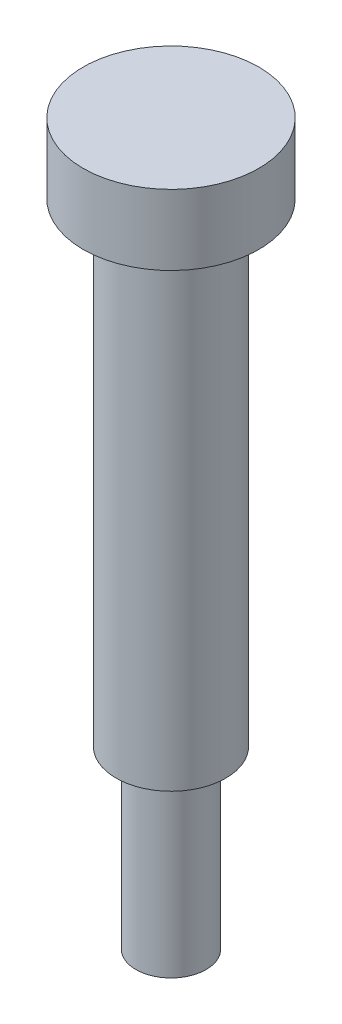
SolidWorks part; units mm, degrees
material "Plain Carbon Steel"
ref_plane "Front Plane" through (0, 0, 0) normal (0, 0, 1) x (1, 0, 0)
ref_plane "Top Plane" through (0, 0, 0) normal (0, 1, 0) x (1, 0, 0)
ref_plane "Right Plane" through (0, 0, 0) normal (1, 0, 0) x (0, 0, -1)
sketch "Screw Profile Sketch" plane through (0, 0, 0) normal (0, 0, 1) x (1, 0, 0)
  line L0 (0, 0) -> (-2, 0)
  line L1 (-2, 0) -> (-2, 10)
  line L2 (-2, 10) -> (-3.125, 10)
  line L3 (-3.125, 10) -> (-3.125, 37)
  line L4 (-3.125, 37) -> (-5, 37)
  line L5 (-5, 41) -> (-5, 37)
  line L6 (0, 0) -> (0, 41)
  line L7 (0, 41) -> (-5, 41)
  line L8 (0, 0) -> (0, 58.2182) construction
  dimension "D1" = 4
  dimension "D2" = 37
  dimension "D3" = 27
  dimension "D4" = 2
  dimension "D5" = 3.125
  dimension "D6" = 5
revolve "Screw Body Revolve" add sketch "Screw Profile Sketch" angle 360 about L8
